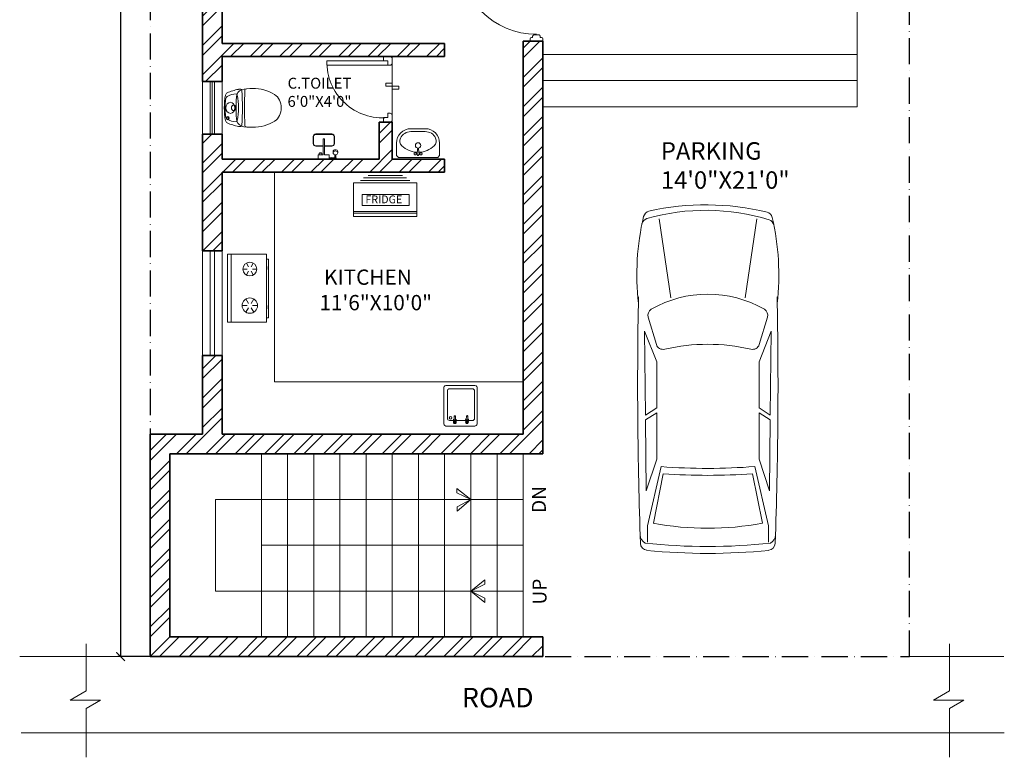
# Model space of a CAD drawing. Units: inches. Extents: x -15 to 1053, y -1 to 793.
# Tile 1 of 8: x -15 to 436, y -1 to 337. Entities that reach past the tile are written whole.
import ezdxf

# ---------------------------------------------------------------- set-up
doc = ezdxf.new("R2010")
doc.units = ezdxf.units.IN
doc.linetypes.add('ACAD_ISO10W100', pattern=[18, 12, -3, 0, -3])
for name, color, linetype, lineweight in [('00 FURNITURE', 15, 'Continuous', 15), ('A-ANNO-DIMS', 2, 'Continuous', 18), ('A-ANNO-SYMB', 2, 'Continuous', 18), ('A-ANNO-TEXT', 7, 'Continuous', 18), ('A-AREA-IDEN', 7, 'Continuous', 18), ('A-DOOR', 4, 'Continuous', 18), ('A-FLOR-CASE', 5, 'Continuous', 18), ('A-FLOR-FIXT', 8, 'Continuous', 13), ('A-FLOR-STRS', 3, 'Continuous', 18), ('A-FURN', 8, 'Continuous', 13), ('A-GLAZ', 4, 'Continuous', 18), ('A-WALL', 7, 'Continuous', 35), ('A-WALL-PATT', 8, 'Continuous', 13), ('A_FUR 1', 5, 'Continuous', 5), ('C-PROP', 1, 'ACAD_ISO10W100', 25), ('C-ROAD', 7, 'Continuous', 18)]:
    doc.layers.add(name, color=color, linetype=linetype, lineweight=lineweight)
doc.layers.add('FURN3D', color=229, linetype='Continuous', lineweight=5, true_color=0x4a3f41)
doc.layers.add('furniture', color=253, linetype='Continuous', lineweight=9, transparency=0.4)
doc.styles.add('1-100DIM', font='txt', dxfattribs={"height": 0.3})
doc.styles.get("Standard").update_dxf_attribs({"font": 'arial.ttf'})
doc.dimstyles.new('ISO-25', dxfattribs={"dimtxt": 8, "dimasz": 4, "dimexe": 1.25, "dimexo": 0.625, "dimtad": 1, "dimdec": 0, "dimlunit": 4, "dimtxsty": 'Standard', "dimblk": 'ARCHTICK', "dimcen": 3, "dimadec": 0, "dimazin": 0, "dimtfac": 1, "dimtdec": 0, "dimtmove": 0, "dimatfit": 3, "dimldrblk": 'ARCHTICK', "dimfxl": 1, "dimarcsym": 0})

# ---------------------------------------------------------------- blocks, each defined once
blk = doc.blocks.new('A$C03CC5C65')
at = {"layer": 'FURN3D'}
for p, q in [((1.56, 18.72, -49.92), (13.66, 18.72, -49.92)), ((0, 0.9, -49.92), (0, 17.82, -49.92)), ((0, 0.9, -29.27), (0, 17.82, -48.65)), ((0, 17.82, -29.27), (0, 0.9, -48.65)), ((4.37, 16.77, -25.9), (4.37, 16.84, -25.9)), ((4.37, 16.77, -25.9), (4.73, 16.4, -25.9)), ((4.37, 15.7, -25.9), (4.73, 16.12, -25.9)), ((4.37, 15.64, -25.9), (4.73, 16.06, -25.9)), ((4.37, 15.64, -25.9), (4.37, 15.7, -25.9)), ((4.48, 16.95, -25.9), (4.87, 16.59, -25.9)), ((4.48, 16.89, -25.9), (4.48, 16.95, -25.9)), ((4.48, 16.89, -25.9), (4.87, 16.52, -25.9)), ((4.48, 15.53, -25.9), (4.87, 15.89, -25.9)), ((4.63, 16.87, -25.9), (4.63, 16.8, -25.9)), ((4.63, 15.67, -25.9), (4.68, 15.67, -25.9)), ((4.63, 15.67), (4.68, 15.67)), ((4.64, 16.49, -25.9), (4.66, 16.05, -25.9)), ((4.83, 16.98, -25.9), (4.68, 16.76, -25.9)), ((4.68, 15.71, -25.9), (4.75, 14.17, -25.9)), ((4.87, 16.91, -25.9), (4.73, 16.71, -25.9)), ((5.24, 16.98, -25.9), (4.83, 16.98, -25.9)), ((4.87, 16.91, -25.9), (4.83, 16.98, -25.9)), ((5.21, 16.91, -25.9), (4.87, 16.91, -25.9)), ((5.21, 16.91, -25.9), (5.24, 16.98, -25.9)), ((5.6, 16.95, -25.9), (5.21, 16.59, -25.9)), ((5.21, 16.91, -25.9), (5.34, 16.71, -25.9)), ((5.6, 16.88, -25.9), (5.21, 16.52, -25.9)), ((5.6, 15.52, -25.9), (5.21, 15.89, -25.9)), ((5.24, 16.98, -25.9), (5.39, 16.76, -25.9)), ((5.39, 15.71, -25.9), (5.32, 14.17, -25.9)), ((5.71, 16.77, -25.9), (5.35, 16.4, -25.9)), ((5.71, 15.7, -25.9), (5.35, 16.12, -25.9)), ((5.71, 15.64, -25.9), (5.35, 16.06, -25.9)), ((5.39, 15.67, -25.9), (5.44, 15.67, -25.9)), ((5.39, 15.67), (5.44, 15.67)), ((5.43, 16.49, -25.9), (5.41, 16.05, -25.9)), ((5.44, 16.87, -25.9), (5.44, 16.8, -25.9)), ((5.6, 16.95, -25.9), (5.6, 16.88, -25.9)), ((5.6, 16.95, -25.9), (5.6, 16.88, -25.9)), ((5.71, 16.77, -25.9), (5.71, 16.83, -25.9)), ((5.71, 15.64, -25.9), (5.71, 15.7, -25.9)), ((9.98, 15.69, -25.9), (10.34, 16.11, -25.9)), ((9.98, 15.63, -25.9), (10.34, 16.05, -25.9)), ((9.98, 15.63, -25.9), (9.98, 15.69, -25.9)), ((9.99, 16.76, -25.9), (9.99, 16.83, -25.9)), ((9.99, 16.76, -25.9), (10.34, 16.39, -25.9)), ((10.09, 16.94, -25.9), (10.48, 16.58, -25.9)), ((10.09, 16.88, -25.9), (10.09, 16.94, -25.9)), ((10.09, 16.88, -25.9), (10.48, 16.51, -25.9)), ((10.09, 15.52, -25.9), (10.48, 15.88, -25.9)), ((10.25, 16.86, -25.9), (10.25, 16.8, -25.9)), ((10.25, 15.66, -25.9), (10.3, 15.66, -25.9)), ((10.25, 15.66), (10.3, 15.66)), ((10.26, 16.47, -25.9), (10.28, 16.03, -25.9)), ((10.45, 16.97, -25.9), (10.3, 16.75, -25.9)), ((10.3, 15.7, -25.9), (10.37, 14.16, -25.9)), ((10.49, 16.9, -25.9), (10.35, 16.7, -25.9)), ((10.86, 16.97, -25.9), (10.45, 16.97, -25.9)), ((10.49, 16.9, -25.9), (10.45, 16.97, -25.9)), ((10.82, 16.9, -25.9), (10.49, 16.9, -25.9)), ((10.82, 16.9, -25.9), (10.86, 16.97, -25.9)), ((11.22, 16.94, -25.9), (10.82, 16.58, -25.9)), ((10.82, 16.9, -25.9), (10.96, 16.7, -25.9)), ((11.22, 16.88, -25.9), (10.82, 16.51, -25.9)), ((11.21, 15.51, -25.9), (10.82, 15.88, -25.9)), ((10.86, 16.97, -25.9), (11.01, 16.75, -25.9)), ((11.01, 15.7, -25.9), (10.93, 14.16, -25.9)), ((11.32, 16.76, -25.9), (10.96, 16.39, -25.9)), ((11.32, 15.69, -25.9), (10.96, 16.11, -25.9)), ((11.32, 15.63, -25.9), (10.96, 16.05, -25.9)), ((11.01, 15.66, -25.9), (11.06, 15.66, -25.9)), ((11.01, 15.66), (11.06, 15.66)), ((11.05, 16.47, -25.9), (11.03, 16.03, -25.9)), ((11.06, 16.86, -25.9), (11.06, 16.8, -25.9)), ((11.22, 16.94, -25.9), (11.22, 16.88, -25.9)), ((11.22, 16.94, -25.9), (11.22, 16.88, -25.9)), ((11.32, 16.76, -25.9), (11.32, 16.83, -25.9)), ((11.32, 15.63, -25.9), (11.32, 15.69, -25.9)), ((15.22, 0.9, -29.27), (15.22, 17.82, -48.65)), ((15.22, 17.82, -29.27), (15.22, 0.9, -48.65)), ((1.56, 0, -28), (13.66, 0, -28))]:
    blk.add_line(p, q, dxfattribs=at)
at = {"layer": 'FURN3D', "elevation": -25.9}
for points in [[(1.61, 15.14), (1.62, 2.5)], [(4.66, 16.1), (2.57, 16.1)], [(10.28, 16.11), (5.41, 16.1)], [(13.12, 16.11), (11.03, 16.11)], [(14.1, 2.52), (14.09, 15.15)], [(2.58, 1.55), (13.13, 1.56)]]:
    blk.add_lwpolyline(points, dxfattribs=at)
at = {"layer": 'FURN3D'}
for centre, radius in [((3.1, 14.9, -25.9), 0.593), ((5.04, 16.22, -25.9), 0.218), ((5.04, 16.87), 0.203), ((5.04, 16.87, -25.9), 0.203), ((10.65, 16.22, -25.9), 0.218), ((10.65, 16.86), 0.203), ((10.65, 16.86, -25.9), 0.203)]:
    blk.add_circle(centre, radius, dxfattribs=at)
at = {"layer": 'FURN3D', "extrusion": (0, 0.814703, 0.579878)}
for centre, start, end in [((-1.56, -49.97, -13.7), 270, 0), ((-13.66, -49.97, -13.7), 180, 270), ((-1.56, -24.37, -16.24), 0, 90), ((-13.66, -24.37, -16.24), 90, 180)]:
    blk.add_arc(centre, 1.56, start, end, dxfattribs=at)
at = {"layer": 'FURN3D', "extrusion": (2.9e-15, -0.814703, 0.579878)}
for centre, start, end in [((1.56, -13.52, -31.49), 90, 180), ((1.56, -39.11, -28.95), 180, 270)]:
    blk.add_arc(centre, 1.56, start, end, dxfattribs=at)
at = {"layer": 'FURN3D', "extrusion": (-2.9e-15, -0.814703, 0.579878)}
for centre, start, end in [((13.66, -13.52, -31.49), 0, 90), ((13.66, -39.11, -28.95), 270, 0)]:
    blk.add_arc(centre, 1.56, start, end, dxfattribs=at)
at = {"layer": 'FURN3D'}
for centre, radius, start, end in [((2.6, 15.1, -25.9), 0.997, 88.2299, 182.3676), ((4.6, 16.73, -25.9), 0.252, 118.1078, 154.1122), ((4.6, 16.66, -25.9), 0.252, 118.1078, 154.1122), ((4.6, 15.75, -25.9), 0.252, 205.7141, 241.7184), ((5.04, 16.87, -25.9), 0.655, 359.2227, 180.6036), ((5.04, 16.88, -25.9), 0.655, 190.8582, 233.614), ((5.04, 16.87, -25.9), 0.406, 359.9131, 179.9131), ((4.54, 16.23, -25.9), 0.25, 317.2189, 42.6074), ((4.54, 16.29, -25.9), 0.25, 317.2189, 352.664), ((5.04, 16.6, -25.9), 0.312, 19.462, 160.6639), ((5.04, 14.37, -25.9), 0.298, 194.8671, 343.5351), ((5.03, 14.18, -25.9), 0.281, 182.7661, 357.0602), ((5.04, 16.24, -25.9), 0.218, 356.8132, 183.0131), ((5.04, 16.77, -25.9), 0.25, 227.2092, 312.6171), ((5.04, 16.71, -25.9), 0.25, 227.2092, 312.6171), ((5.04, 15.7, -25.9), 0.25, 47.2092, 132.6171), ((5.04, 16.44, -25.9), 0.187, 40.218, 139.6082), ((5.53, 16.23, -25.9), 0.25, 137.2189, 222.6074), ((5.53, 16.29, -25.9), 0.25, 187.1622, 222.6074), ((5.04, 16.88, -25.9), 0.655, 306.2123, 348.968), ((5.48, 16.72, -25.9), 0.252, 25.7141, 61.7184), ((5.48, 16.66, -25.9), 0.252, 25.7141, 61.7184), ((5.48, 15.75, -25.9), 0.252, 298.1078, 334.1122), ((10.21, 15.74, -25.9), 0.252, 205.7141, 241.7184), ((10.21, 16.72, -25.9), 0.252, 118.1078, 154.1122), ((10.21, 16.65, -25.9), 0.252, 118.1078, 154.1122), ((10.65, 16.86, -25.9), 0.655, 359.2227, 180.6036), ((10.65, 16.86, -25.9), 0.655, 190.8582, 233.614), ((10.65, 16.86, -25.9), 0.406, 359.9131, 179.9131), ((10.16, 16.22, -25.9), 0.25, 317.2189, 42.6074), ((10.16, 16.28, -25.9), 0.25, 317.2189, 352.664), ((10.66, 16.59, -25.9), 0.312, 19.462, 160.6639), ((10.65, 14.36, -25.9), 0.298, 194.8671, 343.5351), ((10.65, 14.17, -25.9), 0.281, 182.7661, 357.0602), ((10.65, 16.23, -25.9), 0.218, 356.8132, 183.0131), ((10.65, 16.7, -25.9), 0.25, 227.2092, 312.6171), ((10.65, 15.69, -25.9), 0.25, 47.2092, 132.6171), ((10.65, 16.76, -25.9), 0.25, 227.2092, 312.6171), ((10.65, 16.44, -25.9), 0.187, 40.218, 139.6082), ((11.15, 16.22, -25.9), 0.25, 137.2189, 222.6074), ((11.15, 16.28, -25.9), 0.25, 187.1622, 222.6074), ((10.65, 16.86, -25.9), 0.655, 306.2123, 348.968), ((11.1, 15.74, -25.9), 0.252, 298.1078, 334.1122), ((11.1, 16.72, -25.9), 0.252, 25.7141, 61.7184), ((11.1, 16.65, -25.9), 0.252, 25.7141, 61.7184), ((13.09, 15.11, -25.9), 0.997, 357.7426, 91.8802), ((2.61, 2.54, -25.9), 0.997, 177.7426, 271.8802), ((13.1, 2.55, -25.9), 0.997, 268.2299, 2.3676)]:
    blk.add_arc(centre, radius, start, end, dxfattribs=at)
blk = doc.blocks.new('A$C21540130')
at = {"layer": 'FURN3D'}
for p, q in [((1.57, 0), (1.57, 31.11)), ((9.02, 24.29, -27.54), (7.06, 24.29, -27.54)), ((9.61, 25.31), (8.63, 27.01)), ((9.61, 23.27), (8.63, 21.57)), ((10.79, 25.31), (11.77, 27.01)), ((10.79, 23.27), (11.77, 21.57)), ((11.38, 24.29, -27.54), (13.34, 24.29, -27.54)), ((9.61, 8.56), (8.43, 10.6)), ((10.79, 8.56), (11.97, 10.6)), ((9.02, 7.54), (6.67, 7.54)), ((9.61, 6.52), (8.43, 4.48)), ((10.79, 6.52), (11.97, 4.48)), ((11.38, 7.54), (13.73, 7.54))]:
    blk.add_line(p, q, dxfattribs=at)
for points in [[(0, 0), (0, 31.11), (17.9, 31.11), (17.9, 0)], [(18.68, 1.96), (18.68, 28.83), (17.9, 28.83), (17.9, 1.96)]]:
    blk.add_lwpolyline(points, close=True, dxfattribs=at)
for centre, radius in [((10.2, 24.29), 3.14), ((10.2, 7.54), 3.53)]:
    blk.add_circle(centre, radius, dxfattribs=at)
for points in [[(17.9, 24.03), (18.29, 24.03), (17.9, 25.6), (18.29, 25.6)], [(17.9, 6.05), (18.29, 6.05), (17.9, 7.62), (18.29, 7.62)]]:
    blk.add_solid(points, dxfattribs=at)
blk = doc.blocks.new('s_14')
at = {"extrusion": (0, 0, -1)}
for centre, major_axis, start_param, end_param in [((0, -522), (652, 0), 4.476887, 4.947891), ((0, -522), (652, 0), 4.476887, 4.947891), ((681, -279), (914, 0), 3.289642, 3.481728), ((681, -279), (914, 0), 3.289642, 3.481728), ((-143, -45), (39.1, 0), 3.481728, 4.476887), ((-143, -45), (39.1, 0), 3.481728, 4.476887), ((118, -139), (285, 0), 3.130806, 3.616946), ((-125, -42), (19.2, 0), 3.141593, 9.424778), ((-125, -42), (12.2, 0), 3.141593, 9.424778), ((-97, -51), (42.5, 0), 3.616946, 4.577347), ((0, -624), (766, 0), 4.577347, 4.847431), ((0, -74), (67.1, 0), 3.141593, 9.424778), ((0, -113), (32.9, 0), 3.141593, 9.424778), ((97, -51), (42.5, 0), -1.435755, -0.475353), ((-118, -139), (285, 0), -0.475353, 0.010787), ((143, -45), (39.1, 0), -1.335294, -0.340135), ((143, -45), (39.1, 0), -1.335294, -0.340135), ((-682, -278), (914, 0), -0.340135, -0.148049), ((-682, -278), (914, 0), -0.340135, -0.148049), ((999, -342), (1233, -1), 3.141593, 3.282422), ((999, -342), (1233, -1), 3.141593, 3.282422), ((-87, -187), (137, 0), 3.032389, 3.289642), ((-87, -187), (137, 0), 3.032389, 3.289642), ((-207, -197), (16, 0), 1.680926, 3.032389), ((-207, -197), (16, 0), 1.680926, 3.032389), ((-121, -225), (98.7, 0), 3.365215, 4.657014), ((1, 1302), (1900, -1), 1.460666, 1.680926), ((1, 1302), (1900, -1), 1.460666, 1.680926), ((-149, -142), (17.9, 0), 1.839297, 3.130806), ((0, 291), (579, 0), 1.302296, 1.839297), ((-1, -1970), (2282, -1), 4.657014, 4.767764), ((121, -225), (98.7, 0), -1.515421, -0.223622), ((149, -142), (17.9, 0), 0.010787, 1.302296), ((207, -197), (16, 0), 0.109204, 1.460666), ((207, -197), (16, 0), 0.109204, 1.460666), ((-1000, -341), (1233, -1), -0.140829, 0), ((-1000, -341), (1233, -1), -0.140829, 0), ((87, -187), (137, 0), -0.148049, 0.109204), ((87, -187), (137, 0), -0.148049, 0.109204), ((527, -342), (761, 0), 2.693443, 3.141593), ((527, -342), (761, 0), 2.693443, 3.141593), ((-210, -263), (19.7, 0), 3.222651, 4.658459), ((-2, -3376), (3914, -2), 4.658459, 4.766319), ((-527, -341), (761, 0), 0, 0.44815), ((-527, -341), (761, 0), 0, 0.44815), ((210, -263), (19.7, 0), -1.516867, -0.081058), ((0, -544), (176, 0), 0.44815, 2.693443), ((0, -544), (176, 0), 0.44815, 2.693443)]:
    blk.add_ellipse(centre, major_axis=major_axis, ratio=0.800511, start_param=start_param, end_param=end_param, dxfattribs=at)
blk = doc.blocks.new('s_46')
at = {"ltscale": 600}
h = blk.add_hatch(color=256, dxfattribs=at)
edge = h.paths.add_edge_path()
edge.add_line((13, 62), (14, 54))
edge.add_ellipse((4, 52), major_axis=(-10.1, 0), ratio=1, start_angle=540, end_angle=550.1755, ccw=False)
edge.add_arc((4, 52), 10.1, 270, 360, ccw=False)
edge.add_line((4, 42), (4, 41))
edge.add_line((4, 41), (12, 41))
edge.add_arc((4, 52), 13.4, 664.6981, 766.4848)
h.paths.add_polyline_path([(4, 41), (-3, 41, 0.152567), (4, 39)])
h.paths.add_polyline_path([(12, 41), (4, 41), (4, 39, 0.152567)])
h.paths.add_polyline_path([(-6, 54), (-5, 62, 0.475833), (-3, 41), (4, 41), (4, 42, -0.46724)])
for p, q in [((-6, 52), (-1, 110)), ((-6, 52), (-1, 110)), ((9, 110), (14, 54)), ((14, 52), (9, 110)), ((14, 54), (14, 52))]:
    blk.add_line(p, q, dxfattribs=at)
blk.add_lwpolyline([(-221, 171, -0.414214), (-71, 321), (79, 321, -0.414214), (229, 171), (229, 41), (209, 21), (-201, 21), (-221, 41)], format="xyb", close=True, dxfattribs=at)
blk.add_lwpolyline([(12, 75, 0.181638), (172, 142, 0.326351), (188, 223, 0.289814), (79, 291), (-71, 291, 0.289814), (-179, 223, 0.326351), (-164, 142, 0.181638), (-4, 75)], format="xyb", dxfattribs=at)
for points in [[(-17, 67), (-17, 68), (-17, 68), (-17, 68), (-18, 68), (-18, 68), (-18, 68), (-18, 68), (-18, 68), (-18, 68), (-18, 69), (-19, 69), (-19, 69), (-19, 69), (-19, 69), (-19, 69), (-19, 69), (-19, 69), (-20, 69), (-20, 69), (-20, 69), (-20, 69), (-20, 70), (-21, 70), (-21, 70), (-21, 70), (-21, 70), (-21, 70), (-21, 70), (-22, 70), (-22, 71), (-22, 71), (-22, 71), (-22, 71), (-22, 70), (-23, 70), (-23, 70), (-23, 70), (-23, 70), (-23, 70), (-24, 71), (-24, 71), (-24, 71), (-24, 71), (-24, 71), (-25, 71), (-25, 71), (-25, 71), (-25, 71), (-25, 71), (-25, 71), (-26, 71), (-26, 71), (-26, 71), (-26, 71), (-26, 71), (-27, 71), (-27, 71), (-27, 71), (-27, 71), (-27, 71), (-28, 71), (-28, 71), (-28, 71), (-28, 71), (-28, 71), (-29, 71), (-29, 70), (-29, 70), (-29, 70), (-29, 70), (-30, 70), (-30, 70), (-30, 70), (-31, 70), (-31, 70), (-31, 70), (-31, 69), (-32, 68), (-32, 68), (-33, 68), (-33, 68), (-34, 68), (-34, 68), (-34, 68), (-34, 67), (-34, 67), (-34, 67), (-34, 67), (-35, 67), (-35, 66), (-35, 66), (-35, 66), (-35, 66), (-36, 66), (-36, 66), (-36, 66), (-36, 65), (-36, 65), (-36, 65), (-36, 65), (-36, 65), (-36, 64), (-36, 64), (-36, 64), (-36, 64), (-36, 64), (-37, 64), (-37, 64), (-37, 63), (-37, 63), (-37, 63), (-37, 63), (-37, 63), (-37, 63), (-37, 62), (-37, 62), (-37, 62), (-37, 62), (-37, 62), (-37, 61), (-37, 61), (-37, 61), (-38, 61), (-38, 61), (-38, 61), (-38, 60), (-38, 60), (-38, 60), (-38, 60), (-38, 60), (-38, 59), (-37, 59), (-37, 59), (-37, 59), (-37, 59), (-37, 58), (-38, 58), (-38, 58), (-38, 58), (-38, 58), (-38, 57), (-38, 57), (-38, 57), (-38, 57), (-38, 57), (-37, 57), (-37, 56), (-37, 56), (-37, 56), (-37, 56), (-37, 56), (-37, 55), (-37, 55), (-37, 55), (-37, 55), (-37, 55), (-37, 54), (-37, 54), (-37, 54), (-37, 54), (-37, 54), (-36, 54), (-36, 54), (-36, 53), (-36, 53), (-36, 53), (-36, 53), (-36, 53), (-36, 52), (-36, 52), (-36, 52), (-36, 52), (-36, 52), (-36, 52), (-35, 51), (-35, 51), (-35, 51), (-35, 51), (-35, 51), (-34, 51), (-34, 51), (-34, 51), (-34, 51), (-34, 50), (-34, 50), (-34, 50), (-34, 50), (-34, 50), (-34, 49), (-33, 49), (-33, 49), (-33, 49), (-33, 49), (-33, 49), (-32, 49), (-32, 49), (-32, 49), (-32, 49), (-32, 49), (-32, 49), (-31, 48), (-31, 48), (-31, 48), (-31, 48), (-31, 48), (-31, 48), (-31, 48), (-30, 48), (-30, 48), (-30, 48), (-30, 48), (-30, 48), (-29, 48), (-29, 48), (-29, 47), (-29, 47), (-29, 47), (-28, 47), (-28, 47), (-28, 47), (-28, 47), (-28, 47), (-28, 47), (-27, 47), (-27, 47), (-27, 47), (-27, 47), (-27, 47), (-26, 47), (-26, 47), (-26, 47), (-26, 47), (-26, 47), (-25, 47), (-25, 47), (-25, 47), (-25, 46), (-25, 46), (-25, 47), (-24, 47), (-24, 47), (-24, 47), (-24, 47), (-24, 47), (-23, 47), (-23, 47), (-23, 47), (-23, 47), (-23, 47), (-22, 47), (-22, 47), (-22, 47), (-22, 47), (-22, 47), (-22, 47), (-21, 47), (-21, 47), (-21, 48), (-21, 48), (-21, 48), (-21, 48), (-20, 48), (-20, 48), (-20, 48), (-20, 48), (-20, 48), (-19, 48), (-19, 48), (-19, 48), (-19, 48), (-19, 48), (-19, 49), (-19, 49), (-18, 49), (-18, 49), (-18, 49), (-18, 50), (-18, 50), (-18, 50), (-18, 50), (-17, 50), (-17, 50), (-17, 50), (-17, 50), (-17, 50), (-17, 50), (-16, 50), (-16, 51), (-16, 51), (-16, 51), (-16, 51), (-16, 51), (-16, 52), (-16, 52), (-16, 52), (-16, 52), (-15, 52), (-15, 52), (-15, 52), (-15, 53), (-15, 53), (-15, 53), (-15, 53), (-15, 53), (-15, 53), (-15, 54), (-15, 54), (-15, 54), (-15, 54), (-15, 54), (-14, 55), (-14, 55), (-14, 55), (-14, 55), (-14, 55), (-14, 55), (-14, 56), (-14, 56), (-14, 56), (-14, 56), (-14, 56), (-14, 56), (-14, 57), (-14, 57), (-14, 57), (-14, 57), (-14, 57), (-14, 58), (-14, 58), (-13, 58), (-13, 58), (-13, 58), (-13, 59), (-13, 59), (-13, 59), (-13, 59), (-13, 59), (-13, 60), (-14, 60), (-14, 60), (-14, 60), (-14, 60), (-14, 60), (-14, 61), (-14, 61), (-14, 61), (-14, 61), (-14, 61), (-14, 62), (-14, 62), (-14, 62), (-14, 62), (-14, 62), (-14, 62), (-14, 63), (-14, 63), (-14, 63), (-15, 63), (-15, 63), (-15, 64), (-15, 64), (-15, 64), (-15, 64), (-15, 64), (-15, 65), (-15, 65), (-15, 65), (-15, 65), (-15, 65), (-15, 65), (-15, 65), (-16, 65), (-16, 66), (-16, 66), (-16, 66), (-16, 66), (-16, 66), (-16, 67), (-16, 67), (-16, 67), (-16, 67), (-17, 67), (-17, 67)], [(22, 61), (22, 61), (22, 61), (22, 62), (22, 62), (22, 62), (22, 62), (22, 62), (22, 62), (23, 63), (23, 63), (23, 63), (23, 63), (23, 63), (23, 64), (23, 64), (23, 64), (23, 64), (23, 64), (23, 65), (23, 65), (23, 65), (23, 65), (24, 65), (24, 65), (24, 65), (24, 65), (24, 66), (24, 66), (24, 66), (25, 66), (25, 66), (25, 67), (25, 67), (25, 67), (25, 67), (25, 67), (25, 67), (25, 67), (25, 68), (26, 68), (26, 68), (26, 68), (26, 68), (26, 68), (27, 68), (27, 68), (27, 68), (27, 69), (27, 69), (27, 69), (27, 69), (27, 69), (28, 69), (28, 69), (28, 69), (28, 69), (28, 69), (29, 69), (29, 69), (29, 70), (29, 70), (29, 70), (29, 70), (30, 70), (30, 70), (30, 70), (30, 70), (30, 71), (30, 71), (31, 71), (31, 71), (31, 70), (31, 70), (31, 70), (32, 70), (32, 70), (32, 70), (32, 71), (32, 71), (32, 71), (33, 71), (33, 71), (33, 71), (33, 71), (33, 71), (34, 71), (34, 71), (34, 71), (34, 71), (34, 71), (34, 71), (35, 71), (35, 71), (35, 71), (35, 71), (36, 71), (36, 71), (36, 71), (36, 71), (36, 71), (36, 71), (37, 71), (37, 71), (37, 71), (37, 70), (37, 70), (38, 70), (38, 70), (38, 70), (38, 70), (39, 70), (39, 70), (39, 70), (40, 70), (40, 69), (40, 68), (41, 68), (41, 68), (42, 68), (42, 68), (42, 68), (42, 68), (42, 67), (43, 67), (43, 67), (43, 67), (43, 67), (43, 66), (43, 66), (44, 66), (44, 66), (44, 66), (44, 66), (44, 66), (44, 65), (44, 65), (44, 65), (44, 65), (44, 65), (44, 64), (44, 64), (45, 64), (45, 64), (45, 64), (45, 64), (45, 64), (45, 63), (45, 63), (45, 63), (45, 63), (45, 63), (45, 63), (45, 62), (45, 62), (45, 62), (45, 62), (45, 62), (46, 61), (46, 61), (46, 61), (46, 61), (46, 61), (46, 61), (46, 60), (46, 60), (46, 60), (46, 60), (46, 60), (46, 59), (46, 59), (46, 59), (46, 59), (46, 59), (46, 58), (46, 58), (46, 58), (46, 58), (46, 58), (46, 57), (46, 57), (46, 57), (46, 57), (46, 57), (46, 57), (46, 56), (46, 56), (45, 56), (45, 56), (45, 56), (45, 55), (45, 55), (45, 55), (45, 55), (45, 55), (45, 54), (45, 54), (45, 54), (45, 54), (45, 54), (45, 54), (45, 54), (45, 53), (44, 53), (44, 53), (44, 53), (44, 53), (44, 52), (44, 52), (44, 52), (44, 52), (44, 52), (44, 52), (44, 51), (44, 51), (43, 51), (43, 51), (43, 51), (43, 51), (43, 51), (43, 51), (42, 51), (42, 50), (42, 50), (42, 50), (42, 50), (42, 50), (42, 49), (42, 49), (42, 49), (41, 49), (41, 49), (41, 49), (41, 49), (41, 49), (40, 49), (40, 49), (40, 49), (40, 49), (40, 48), (40, 48), (40, 48), (39, 48), (39, 48), (39, 48), (39, 48), (39, 48), (39, 48), (38, 48), (38, 48), (38, 48), (38, 48), (38, 48), (37, 47), (37, 47), (37, 47), (37, 47), (37, 47), (37, 47), (36, 47), (36, 47), (36, 47), (36, 47), (36, 47), (36, 47), (35, 47), (35, 47), (35, 47), (35, 47), (34, 47), (34, 47), (34, 47), (34, 47), (34, 47), (34, 47), (33, 46), (33, 46), (33, 47), (33, 47), (33, 47), (32, 47), (32, 47), (32, 47), (32, 47), (32, 47), (32, 47), (31, 47), (31, 47), (31, 47), (31, 47), (31, 47), (30, 47), (30, 47), (30, 47), (30, 47), (30, 47), (30, 48), (29, 48), (29, 48), (29, 48), (29, 48), (29, 48), (29, 48), (28, 48), (28, 48), (28, 48), (28, 48), (28, 48), (27, 48), (27, 48), (27, 49), (27, 49), (27, 49), (27, 49), (27, 49), (27, 50), (26, 50), (26, 50), (26, 50), (26, 50), (26, 50), (25, 50), (25, 50), (25, 50), (25, 50), (25, 50), (25, 51), (25, 51), (25, 51), (25, 51), (25, 51), (24, 52), (24, 52), (24, 52), (24, 52), (24, 52), (24, 52), (24, 52), (23, 53), (23, 53), (23, 53), (23, 53), (23, 53), (23, 53), (23, 54), (23, 54), (23, 54), (23, 54), (23, 54), (23, 55), (23, 55), (23, 55), (22, 55), (22, 55), (22, 55), (22, 56), (22, 56), (22, 56), (22, 56), (22, 56), (22, 56), (22, 57), (22, 57), (22, 57), (22, 57), (22, 57), (22, 58), (22, 58), (22, 58), (22, 58), (22, 58), (22, 59), (22, 59), (22, 59), (22, 59), (22, 59), (22, 60), (22, 60), (22, 60), (22, 60), (22, 60), (22, 60), (22, 61), (22, 61)]]:
    blk.add_lwpolyline(points, close=True, dxfattribs=at)
blk.add_circle((4, 146), 28, dxfattribs=at)
for centre, radius, start, end in [((4, 108), 5.42, 24.6783, 155.3217), ((4, 52), 10.1, 169.8245, 0)]:
    blk.add_arc(centre, radius, start, end, dxfattribs=at)
for centre, major_axis, ratio, start_param, end_param in [((4, 110), (-4.93, 0), 0.641024, 3.141593, 6.283185), ((4, 52), (-10.1, 0), 1, 6.10559, 9.602373)]:
    blk.add_ellipse(centre, major_axis=major_axis, ratio=ratio, start_param=start_param, end_param=end_param, dxfattribs=at)
blk = doc.blocks.new('A$C7A0926BE')
for p, q in [((-6.55, 0), (-5.57, 0)), ((-6.55, -0.65), (-6.55, 0)), ((-5.57, 0), (-5.57, -0.65)), ((-2.89, 0), (-2.89, -2.29)), ((2.89, 0), (-2.89, 0)), ((2.89, -2.29), (2.89, 0)), ((-7.32, -3.29), (-7.32, -3.94)), ((-5.57, -0.65), (-6.55, -0.65)), ((-6.34, -0.65), (-5.74, -0.65)), ((-6.34, -2.33), (-6.34, -0.65)), ((-5.74, -2.33), (-6.34, -2.33)), ((-5.74, -0.65), (-5.74, -2.33)), ((-5.57, -0.28), (-2.89, -0.56)), ((-5.57, -0.65), (-2.89, -0.94)), ((-4.84, -3.94), (-4.85, -3.29)), ((-2.89, -2.29), (-0.45, -2.29)), ((0.39, -2.29), (2.89, -2.29)), ((1.04, -2.29), (1.04, -3.12)), ((2.37, -2.29), (1.04, -2.29)), ((1.04, -3.12), (2.37, -3.12)), ((1.13, -3.12), (1.13, -3.23)), ((2.3, -3.12), (1.13, -3.12)), ((1.13, -3.23), (2.3, -3.23)), ((2.3, -3.23), (2.3, -3.12)), ((2.37, -3.12), (2.37, -2.29))]:
    blk.add_line(p, q)
at = {"ltscale": 100}
for p, q in [((-0.45, -10.48), (-0.45, -2.29)), ((0.39, -10.48), (0.39, -2.29)), ((0.18, -10.69), (-0.24, -10.69))]:
    blk.add_line(p, q, dxfattribs=at)
for points in [[(-0.45, -6.79), (-4.23, -6.79, 0.414214), (-5.63, -8.19), (-5.63, -11.8, 0.414214), (-4.23, -13.2), (4.17, -13.2, 0.414214), (5.57, -11.8), (5.57, -8.19, 0.414214), (4.17, -6.79), (0.39, -6.79)], [(-0.45, -7), (-4.23, -7, 0.414214), (-5.42, -8.19), (-5.42, -11.8, 0.414214), (-4.23, -12.99), (4.17, -12.99, 0.414214), (5.36, -11.8), (5.36, -8.19, 0.414214), (4.17, -7), (0.39, -7)]]:
    blk.add_lwpolyline(points, format="xyb", dxfattribs=at)
for centre, start, end in [((-0.24, -10.48), 180, 270), ((0.18, -10.48), 270, 0)]:
    blk.add_arc(centre, 0.21, start, end, dxfattribs=at)
at = {"extrusion": (0, 0, -1)}
blk.add_ellipse((-6.08, -3.29), major_axis=(-1.24, 0), ratio=0.790849, dxfattribs=at)
blk.add_ellipse((-6.08, -3.94), major_axis=(-1.24, 0), ratio=0.790849, start_param=3.141593, end_param=6.283185, dxfattribs=at)
blk = doc.blocks.new('DDD')
at = {"layer": '00 FURNITURE'}
for p, q in [((-12579.77, -15859.53), (-12579.77, -15829.05)), ((-12578.77, -15859.53), (-12578.77, -15829.03)), ((-12612.02, -15857.03), (-12612.02, -15862.03)), ((-12611.02, -15857.03), (-12612.02, -15857.03)), ((-12610.52, -15858.03), (-12610.52, -15857.53)), ((-12577.52, -15858.03), (-12577.52, -15857.53)), ((-12577.02, -15857.03), (-12576.02, -15857.03)), ((-12576.02, -15857.03), (-12576.02, -15862.03)), ((-12610.52, -15861.53), (-12610.52, -15861.03)), ((-12578.77, -15859.53), (-12579.77, -15859.53)), ((-12577.52, -15861.53), (-12577.52, -15861.03)), ((-12612.02, -15862.03), (-12611.02, -15862.03)), ((-12576.02, -15862.03), (-12577.02, -15862.03))]:
    blk.add_line(p, q, dxfattribs=at)
for points in [[(-12610.52, -15861.03), (-12610.02, -15861.03, 0.414214), (-12609.52, -15860.53), (-12609.52, -15858.53, 0.414214), (-12610.02, -15858.03), (-12610.52, -15858.03)], [(-12577.52, -15861.03), (-12578.02, -15861.03, -0.414214), (-12578.52, -15860.53), (-12578.52, -15858.53, -0.414214), (-12578.02, -15858.03), (-12577.52, -15858.03)]]:
    blk.add_lwpolyline(points, format="xyb", dxfattribs=at)
for centre, radius, start, end in [((-12578.77, -15859.53), 30.5, 90, 180), ((-12611.02, -15857.53), 0.5, 0, 90), ((-12577.02, -15857.53), 0.5, 90, 180), ((-12611.02, -15861.53), 0.5, 270, 0), ((-12577.02, -15861.53), 0.5, 180, 270)]:
    blk.add_arc(centre, radius, start, end, dxfattribs=at)
blk = doc.blocks.new('A$C5BBA3387')
at = {"layer": 'furniture'}
for p, q in [((16.49, 29.07), (16.49, 0)), ((17.22, 29.07), (17.22, 0)), ((1.08, 24.37), (1.08, 4.58)), ((2.29, 25.81), (2.29, 3.26)), ((0, 22.44), (0, 6.75))]:
    blk.add_line(p, q, dxfattribs=at)
for points in [[(18.78, 29.07), (18.78, 0), (3.37, 0), (3.37, 29.07)], [(8.63, 4.02), (8.63, 25.56), (13.78, 25.56), (13.78, 4.02)]]:
    blk.add_lwpolyline(points, close=True, dxfattribs=at)
at = {"layer": 'furniture', "insert": (9.12, 5.47), "char_height": 3.589, "width": 57.8029, "attachment_point": 1, "rotation": 90}
blk.add_mtext('FRIDGE', dxfattribs=at)
blk = doc.blocks.new('_ArchTick')
at = {"color": 0, "linetype": 'ByBlock', "const_width": 0.15}
blk.add_lwpolyline([(-0.5, -0.5), (0.5, 0.5)], dxfattribs=at)
blk = doc.blocks.new('*D17')
at = {"layer": 'A-ANNO-DIMS', "color": 0, "lineweight": -2, "transparency": 16777216}
for p, q in [((44.24, 764.76), (30.11, 764.76)), ((31.36, 764.76), (31.36, 44.76)), ((44.24, 44.76), (30.11, 44.76))]:
    blk.add_line(p, q, dxfattribs=at)
at = {"layer": 'Defpoints', "color": 0, "transparency": 16777216}
for p in [(44.87, 764.76), (31.36, 44.76), (44.87, 44.76)]:
    blk.add_point(p, dxfattribs=at)
at = {"layer": 'A-ANNO-DIMS', "color": 0, "lineweight": -2, "transparency": 16777216, "xscale": 4, "yscale": 4, "zscale": 4}
for p, rotation in [((31.36, 764.76), 90), ((31.36, 44.76), 270)]:
    blk.add_blockref('_ArchTick', p, dxfattribs=dict(at, rotation=rotation))
at = {"layer": 'A-ANNO-DIMS', "color": 0, "transparency": 16777216, "insert": (26.65, 404.76), "char_height": 8, "attachment_point": 5, "rotation": 90}
blk.add_mtext("60'", dxfattribs=at)
blk = doc.blocks.new('ESTSET')
at = {"layer": 'A_FUR 1'}
for p, q in [((-10.44, 4.1), (-10.44, 32.1)), ((-8.44, 4.1), (-8.44, 32.1)), ((-36.44, 6.1), (-36.44, 3.1)), ((-34.44, 6.1), (-36.44, 6.1)), ((-34.44, 4.1), (-34.44, 6.1)), ((-34.44, 4.1), (-34.44, 6.1)), ((-8.44, 4.1), (-8.44, 6.1)), ((-8.44, 6.1), (-6.44, 6.1)), ((-8.44, 4.1), (-8.44, 6.1)), ((-6.44, 6.1), (-6.44, 3.1)), ((-6.44, 2.1), (-36.44, 2.1)), ((-35.44, 2.1), (-33.44, 2.1)), ((-32.44, 4.1), (-34.44, 4.1)), ((-32.44, 4.1), (-34.44, 4.1)), ((-32.44, 3.1), (-32.44, 4.1)), ((-10.44, 3.1), (-10.44, 4.1)), ((-10.44, 4.1), (-8.44, 4.1)), ((-10.44, 4.1), (-8.44, 4.1)), ((-7.44, 2.1), (-9.44, 2.1))]:
    blk.add_line(p, q, dxfattribs=at)
for points in [[(-21.44, 2.1), (-18.67, 2.1), (-18.67, 5.1), (-20.06, 5.1)], [(-20.06, 5.1), (-20.06, -0.91)], [(-21.44, 2.1), (-21.44, -0.91), (-20.06, -0.91)]]:
    blk.add_lwpolyline(points, dxfattribs=at)
for centre, radius, start, end in [((-8.91, 6.46), 25.64, 88.9606, 185.2816), ((-35.44, 3.1), 1, 180, 270), ((-33.44, 3.1), 1, 270, 0), ((-9.44, 3.1), 1, 180, 270), ((-7.44, 3.1), 1, 270, 0)]:
    blk.add_arc(centre, radius, start, end, dxfattribs=at)
blk = doc.blocks.new('BREAK-SYMBOL')
for p, q in [((7.31, 51.97), (7.31, 30.42)), ((7.31, 30.42), (0, 26.2)), ((0, 26.2), (13.84, 26.2)), ((13.84, 26.2), (7.31, 22.43)), ((7.31, 22.43), (7.31, 0))]:
    blk.add_line(p, q)

msp = doc.modelspace()

# ---------------------------------------------------------------- hatches: boundary and pattern name
at = {"layer": 'A-WALL-PATT'}
h = msp.add_hatch(dxfattribs=at)
h.set_pattern_fill('ANSI32', color=256)
h.paths.add_polyline_path([(266.87, 740.76), (68.87, 740.76), (68.87, 695.76), (77.87, 695.76), (77.87, 731.76), (215.87, 731.76), (215.87, 647.76), (221.87, 647.76), (221.87, 731.76), (266.87, 731.76)])
h.paths.add_polyline_path([(368.87, 740.76), (314.87, 740.76), (314.87, 731.76), (359.87, 731.76), (359.87, 695.76), (368.87, 695.76)])
h.paths.add_polyline_path([(368.87, 647.76), (359.87, 647.76), (359.87, 611.76), (257.87, 611.76), (257.87, 605.76), (281.87, 605.76), (281.87, 587.76), (287.87, 587.76), (287.87, 605.76), (359.87, 605.76), (359.87, 593.76), (368.87, 593.76)])
h.paths.add_polyline_path([(245.87, 377.76), (221.87, 377.76), (221.87, 611.76), (216.87, 611.76), (77.87, 611.76), (77.87, 647.76), (68.87, 647.76), (68.87, 605.76), (215.87, 605.76), (215.87, 475.76), (191.87, 475.76), (191.87, 469.76), (215.87, 469.76), (215.87, 368.76), (245.87, 368.76)])
h.paths.add_polyline_path([(368.87, 503.76), (359.87, 503.76), (359.87, 368.76), (368.87, 368.76)])
h.paths.add_polyline_path([(368.87, 569.76), (359.87, 569.76), (359.87, 557.76), (257.87, 557.76), (257.87, 551.76), (368.87, 551.76)])
h.paths.add_polyline_path([(155.87, 475.76), (77.87, 475.76), (77.87, 569.76), (68.87, 569.76), (68.87, 469.76), (155.87, 469.76)])
h.paths.add_polyline_path([(77.87, 319.76), (179.87, 319.76), (179.87, 325.76), (77.87, 325.76), (77.87, 421.76), (68.87, 421.76), (68.87, 308.26), (77.87, 308.26)])
h.paths.add_polyline_path([(77.87, 266.76), (179.87, 266.76), (179.87, 272.76), (155.87, 272.76), (155.87, 289.76), (149.87, 289.76), (149.87, 272.76), (77.87, 272.76), (77.87, 284.26), (68.87, 284.26), (68.87, 230.76), (77.87, 230.76)], flags=17)
h.paths.add_polyline_path([(224.87, 326.76), (215.87, 326.76), (215.87, 146.76), (77.87, 146.76), (77.87, 182.76), (68.87, 182.76), (68.87, 146.76), (44.87, 146.76), (44.87, 44.76), (224.87, 44.76), (224.87, 53.76), (53.87, 53.76), (53.87, 137.76), (224.87, 137.76)])

# ---------------------------------------------------------------- linework, layer by layer
at = {"layer": 'A-FLOR-CASE'}
for p, q in [((101.87, 266.76), (101.87, 170.76)), ((101.87, 170.76), (215.87, 170.76))]:
    msp.add_line(p, q, dxfattribs=at)
at = {"layer": 'A-FLOR-STRS'}
for p, q in [((368.87, 368.76), (368.87, 296.76)), ((368.87, 320.76), (224.87, 320.76)), ((368.87, 308.76), (224.87, 308.76)), ((368.87, 296.76), (224.87, 296.76)), ((95.87, 137.76), (95.87, 53.76)), ((107.87, 137.76), (107.87, 53.76)), ((119.87, 137.76), (119.87, 53.76)), ((131.87, 137.76), (131.87, 53.76)), ((143.87, 137.76), (143.87, 53.76)), ((155.87, 137.76), (155.87, 53.76)), ((167.87, 137.76), (167.87, 53.76)), ((179.87, 137.76), (179.87, 53.76)), ((191.87, 137.76), (191.87, 53.76)), ((203.87, 137.76), (203.87, 53.76)), ((215.87, 137.76), (215.87, 53.76)), ((95.87, 95.76), (215.87, 95.76)), ((191.87, 74.76), (198.25, 69.56)), ((198.25, 71.55), (191.87, 74.76)), ((198.25, 69.56), (198.25, 71.55))]:
    msp.add_line(p, q, dxfattribs=at)
for points in [[(185.43, 119.88), (191.87, 116.76), (185.4, 121.87)], [(185.53, 113.46), (191.87, 116.76), (185.56, 111.47)], [(198.25, 79.96), (198.25, 77.97), (191.87, 74.76)]]:
    msp.add_lwpolyline(points, close=True, dxfattribs=at)
msp.add_lwpolyline([(215.87, 74.76), (74.87, 74.76), (74.87, 116.7), (215.87, 116.7)], dxfattribs=at)
at = {"layer": 'A-FURN'}
for p, q in [((278.22, 245.41), (283.55, 209.17)), ((322.94, 245.41), (317.61, 209.17)), ((273.16, 200.29), (276.92, 187.84)), ((327.79, 200.29), (324.03, 187.84)), ((271.46, 193.91), (277.04, 179.85)), ((271.93, 155.45), (271.46, 193.91)), ((329.56, 193.91), (323.98, 179.85)), ((329.08, 155.45), (329.56, 193.91)), ((277.04, 179.85), (277.04, 158.81)), ((323.98, 179.85), (323.98, 158.81)), ((277.04, 158.81), (271.93, 155.45)), ((323.98, 158.81), (329.08, 155.45)), ((277.04, 156.55), (271.96, 153.22)), ((277.04, 156.55), (277.04, 135.3)), ((323.98, 156.55), (323.98, 135.3)), ((323.98, 156.55), (329.05, 153.22)), ((272.21, 120.75), (271.96, 153.22)), ((328.8, 120.75), (329.05, 153.22)), ((277.04, 135.3), (272.21, 120.75)), ((279.08, 131.85), (272.83, 104.69)), ((322.02, 131.86), (328.27, 104.69)), ((323.98, 135.3), (328.8, 120.75)), ((275.53, 105.85), (280.05, 128.58)), ((325.48, 105.85), (320.97, 128.58)), ((272.83, 104.69), (272.83, 97.23)), ((328.27, 104.69), (328.27, 97.23))]:
    msp.add_line(p, q, dxfattribs=at)
for centre, radius, start, end in [((274.31, 245.68), 3.34, 104.3452, 166.6607), ((299.61, 150.03), 99.28, 73.0347, 105.8141), ((299.61, 132.67), 119.14, 76.3976, 102.667), ((326.74, 245.25), 3.34, 13.1156, 74.5941), ((383.41, 219.81), 115.47, 166.6607, 186.5655), ((273.58, 242.36), 3.34, 107.8179, 168.3942), ((327.48, 241.83), 3.34, 11.3249, 70.8826), ((217.54, 219.81), 115.47, 353.4345, 13.1156), ((2341.42, 169.46), 2073.11, 178.89024, 182.01225), ((300.47, 158.93), 51.94, 60.0774, 119.9226), ((-1740.47, 169.46), 2073.11, 357.98775, 1.10976), ((276.22, 201.21), 3.2, 121.1455, 196.7984), ((324.73, 201.21), 3.2, 343.2016, 58.8545), ((279.98, 188.76), 3.2, 196.7984, 283.6631), ((300.47, 99.68), 88.22, 77.0683, 102.9317), ((320.97, 188.76), 3.2, 256.3369, 343.2016), ((300.47, 409.29), 278.26, 265.5919, 274.4407), ((300.47, 407.48), 279.65, 265.7971, 274.2029), ((300.47, 243.31), 139.72, 259.6897, 280.3103), ((274.34, 100.88), 4.9, 184.3987, 237.5288), ((326.61, 100.88), 4.9, 302.4712, 355.6013), ((272.93, 96.79), 3.34, 182.1119, 263.4899), ((300.47, 371.1), 275.86, 264.0142, 275.9858), ((328.02, 96.79), 3.34, 276.5101, 357.8881), ((300.47, 370.02), 277.96, 264.2342, 275.7658)]:
    msp.add_arc(centre, radius, start, end, dxfattribs=at)
at = {"layer": 'A-GLAZ'}
for p, q in [((72.37, 284.26), (72.37, 308.26)), ((73.37, 284.26), (73.37, 308.26)), ((74.37, 284.26), (74.37, 308.26)), ((68.87, 230.76), (68.87, 182.76)), ((72.37, 230.76), (72.37, 182.76)), ((74.37, 230.76), (74.37, 182.76)), ((77.87, 230.76), (77.87, 182.76))]:
    msp.add_line(p, q, dxfattribs=at)
msp.add_lwpolyline([(77.87, 308.26), (68.87, 308.26), (68.87, 284.26), (77.87, 284.26)], close=True, dxfattribs=at)
at = {"layer": 'A-WALL'}
for p, q in [((68.87, 421.76), (68.87, 308.26)), ((77.87, 421.76), (77.87, 325.76)), ((179.87, 325.76), (77.87, 325.76)), ((179.87, 325.76), (179.87, 319.76)), ((224.87, 326.76), (215.87, 326.76)), ((215.87, 326.76), (215.87, 146.76)), ((224.87, 326.76), (224.87, 137.76)), ((179.87, 319.76), (77.87, 319.76)), ((77.87, 319.76), (77.87, 308.26)), ((77.87, 308.26), (68.87, 308.26)), ((149.87, 289.76), (149.87, 272.76)), ((155.87, 289.76), (149.87, 289.76)), ((155.87, 289.76), (155.87, 272.76)), ((77.87, 284.26), (68.87, 284.26)), ((68.87, 284.26), (68.87, 230.76)), ((77.87, 284.26), (77.87, 272.76)), ((77.87, 272.76), (149.87, 272.76)), ((155.87, 272.76), (179.87, 272.76)), ((179.87, 272.76), (179.87, 266.76)), ((77.87, 266.76), (179.87, 266.76)), ((77.87, 266.76), (77.87, 230.76)), ((77.87, 230.76), (68.87, 230.76)), ((77.87, 182.76), (68.87, 182.76)), ((68.87, 182.76), (68.87, 146.76)), ((77.87, 182.76), (77.87, 146.76)), ((44.87, 146.76), (68.87, 146.76)), ((44.87, 146.76), (44.87, 44.76)), ((77.87, 146.76), (215.87, 146.76)), ((53.87, 137.76), (224.87, 137.76)), ((53.87, 137.76), (53.87, 53.76)), ((53.87, 53.76), (224.87, 53.76)), ((224.87, 53.76), (224.87, 44.76)), ((44.87, 44.76), (224.87, 44.76))]:
    msp.add_line(p, q, dxfattribs=at)
at = {"layer": 'C-PROP'}
for p, q in [((44.87, 764.76), (44.87, 44.76)), ((392.87, 44.76), (392.87, 764.76)), ((44.87, 44.76), (392.87, 44.76))]:
    msp.add_line(p, q, dxfattribs=at)
at = {"layer": 'C-ROAD'}
for p, q in [((44.87, 44.76), (-14.88, 44.76)), ((392.87, 44.76), (436.21, 44.76)), ((-14.26, 9.83), (436.35, 9.83))]:
    msp.add_line(p, q, dxfattribs=at)

# ---------------------------------------------------------------- block references
at = {"layer": 'A-ANNO-SYMB'}
for p in [(8.31, -1.39), (403.96, -1.39)]:
    msp.add_blockref('BREAK-SYMBOL', p, dxfattribs=at)
at = {"layer": 'A-DOOR', "xscale": 1.166666666666136, "yscale": 1.166666666666136, "zscale": 1.166666666666136, "rotation": 90}
msp.add_blockref('DDD', (-18280.83, 15040.79), dxfattribs=at)
at = {"layer": 'A-DOOR'}
for name, p, rotation in [('ESTSET', (157.96, 326.21), 90.00000000000003), ('A$C5BBA3387', (138.09, 265.22), 270)]:
    msp.add_blockref(name, p, dxfattribs=dict(at, rotation=rotation))
at = {"layer": 'A-FLOR-FIXT', "xscale": 0.0381558672165204, "yscale": 0.0381558672165204, "zscale": 0.0381558672165204, "rotation": 89.99999999999999}
msp.add_blockref('s_14', (78.87, 296.26), dxfattribs=at)
at = {"layer": 'A-FLOR-FIXT', "extrusion": (0, 0, -1), "xscale": -0.8732967133751344, "yscale": 0.8732967133751344, "zscale": -0.8732967133751344, "rotation": 180}
msp.add_blockref('A$C7A0926BE', (-124.48, 272.76), dxfattribs=at)
at = {"layer": 'A-FLOR-FIXT', "xscale": 0.0438792252617072, "yscale": 0.0438792252617072, "zscale": 0.0438792252617072}
msp.add_blockref('s_46', (167.5, 272.61), dxfattribs=at)
at = {"layer": 'A-FLOR-FIXT'}
msp.add_blockref('A$C21540130', (80.39, 198.09), dxfattribs=at)
at = {"layer": 'A-FLOR-FIXT', "xscale": -1, "rotation": 180}
msp.add_blockref('A$C03CC5C65', (179.5, 169.08, 49.92), dxfattribs=at)

# ---------------------------------------------------------------- texts
at = {"layer": 'A-ANNO-TEXT', "char_height": 6.4099, "attachment_point": 3, "rotation": 90, "style": '1-100DIM'}
for s, insert in [('\\pxqc;{\\f@Malgun Gothic|b0|i0|c0|p34;DN}', (219.86, 139.01)), ('\\pxqc;{\\f@Malgun Gothic|b0|i0|c0|p34;UP}', (220.14, 96.8))]:
    msp.add_mtext_dynamic_manual_height_columns(s, width=44.4859, gutter_width=15.85, heights=[0], dxfattribs=dict(at, insert=insert))
at = {"layer": 'A-ANNO-TEXT', "insert": (187.8, 30.45), "char_height": 9, "attachment_point": 1}
msp.add_mtext_dynamic_manual_height_columns('ROAD', width=36.3273, gutter_width=12.5, heights=[0], dxfattribs=at)
at = {"layer": 'A-AREA-IDEN', "attachment_point": 1, "style": '1-100DIM'}
for s, insert, char_height in [('\\pxqc;{\\f@Malgun Gothic|b0|i0|c0|p34;C.TOILET\\P6\'0"X4\'0"}', (72.65, 310.05), 5), ('{\\f@Malgun Gothic|b0|i0|c0|p34;   KITCHEN\\P  11\'6"X10\'0"}', (118.18, 222.16), 7)]:
    msp.add_mtext_dynamic_manual_height_columns(s, width=99.7063, gutter_width=15.85, heights=[0], dxfattribs=dict(at, insert=insert, char_height=char_height))
at = {"layer": 'A-AREA-IDEN', "insert": (278.96, 280.51), "char_height": 8, "attachment_point": 1}
msp.add_mtext_dynamic_manual_height_columns('PARKING\\P14\'0"X21\'0"', width=80.2451, gutter_width=12.5, heights=[0], dxfattribs=at)

# ---------------------------------------------------------------- dimensions: what is measured, and where the dimension line sits
at = {"layer": 'A-ANNO-DIMS'}
dim = msp.add_linear_dim(base=(31.36, 44.76), p1=(44.87, 764.76), p2=(44.87, 44.76), angle=90, dimstyle='ISO-25', override={"dimclrd": 0, "dimclre": 0, "dimclrt": 0}, dxfattribs=at)
dim.commit()
dim.dimension.update_dxf_attribs({"geometry": '*D17', "text_midpoint": (26.65, 404.76)})

doc.saveas('drawing.dxf')
